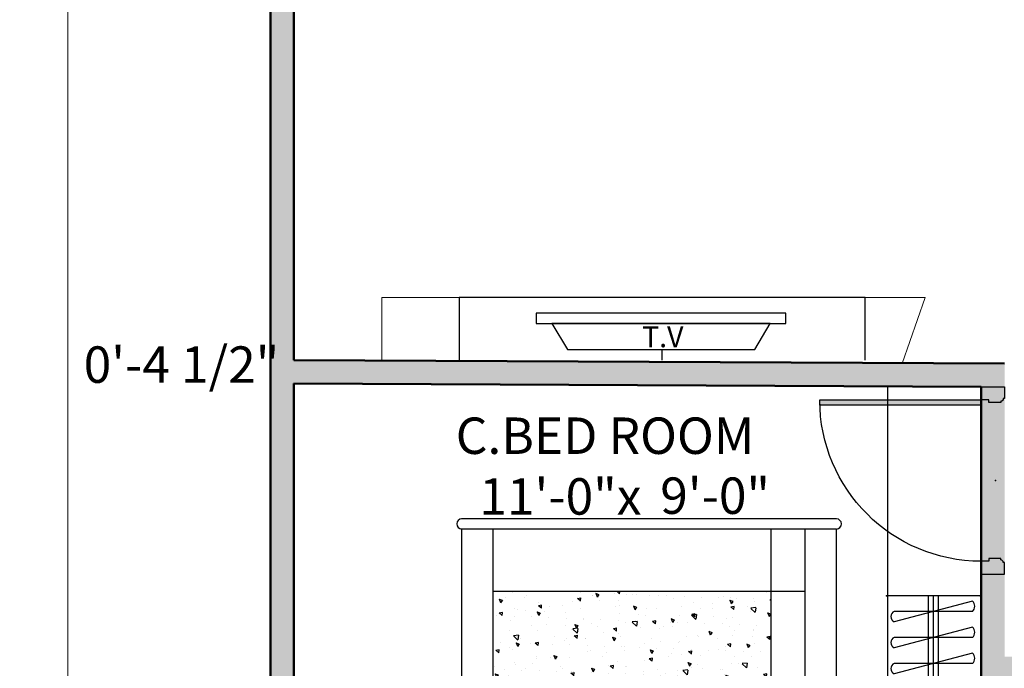
# Model space of a CAD drawing. Units: inches. Extents: x 4508 to 5907, y 877 to 1592.
# Tile 9 of 20: x 5203 to 5392, y 1049 to 1174. Entities that reach past the tile are written whole.
import ezdxf

# ---------------------------------------------------------------- set-up
doc = ezdxf.new("R2010")
doc.units = ezdxf.units.IN
doc.layers.get('DEFPOINTS').update_dxf_attribs({"color": 8})
for name, color, linetype, lineweight in [('A-ANNO-DIMS', 2, 'Continuous', 18), ('A-DOOR', 4, 'Continuous', 25), ('A-FLOR-CASE', 30, 'Continuous', 25), ('A-FURN', 24, 'Continuous', 18), ('A-WALL', 7, 'Continuous', 50), ('A-WALL-PATT', 8, 'Continuous', 13)]:
    doc.layers.add(name, color=color, linetype=linetype, lineweight=lineweight)
doc.layers.add('doors & windows', color=30, linetype='Continuous')
doc.layers.add('furniture', color=24, linetype='Continuous')
doc.styles.get("Standard").update_dxf_attribs({"font": 'arial.ttf'})
doc.dimstyles.new('details', dxfattribs={"dimtxt": 5, "dimasz": 2, "dimexe": 2, "dimexo": 3, "dimgap": 1, "dimtad": 0, "dimdec": 1, "dimzin": 0, "dimdsep": 46, "dimlunit": 4, "dimtxsty": 'Standard', "dimblk": 'ARCHTICK', "dimcen": 3, "dimclrd": 256, "dimclre": 256, "dimclrt": 256, "dimadec": 0, "dimazin": 0, "dimtfac": 0.5, "dimtdec": 1, "dimtofl": 0, "dimtmove": 0, "dimatfit": 3, "dimldrblk": 'CLOSEDBLANK', "dimfxl": 2, "dimtolj": 1, "dimtzin": 0, "dimlwd": -1, "dimlwe": -1, "dimarcsym": 0})
doc.dimstyles.new('text', dxfattribs={"dimtxt": 7, "dimasz": 0, "dimexe": 3, "dimexo": 3, "dimgap": 0, "dimtad": 1, "dimtih": 1, "dimtoh": 1, "dimzin": 3, "dimdsep": 46, "dimlunit": 4, "dimtxsty": 'Standard', "dimblk": 'CLOSEDBLANK', "dimcen": 3, "dimse1": 1, "dimse2": 1, "dimsd1": 1, "dimsd2": 1, "dimclrd": 256, "dimclre": 256, "dimclrt": 256, "dimadec": 0, "dimazin": 0, "dimtfac": 0.5, "dimtofl": 0, "dimtmove": 0, "dimatfit": 3, "dimfxl": 3, "dimtolj": 1, "dimtzin": 0, "dimlwd": -1, "dimlwe": -1, "dimarcsym": 0})

# ---------------------------------------------------------------- blocks, each defined once
blk = doc.blocks.new('_ArchTick')
at = {"color": 0, "linetype": 'ByBlock', "const_width": 0.15}
blk.add_lwpolyline([(-0.5, -0.5), (0.5, 0.5)], dxfattribs=at)
blk = doc.blocks.new('*D77')
at = {"layer": 'A-ANNO-DIMS', "color": 0, "transparency": 16777216}
for p, q in [((5201.49, 1574.7), (5213.97, 1574.7)), ((5211.97, 1574.7), (5211.97, 1255.95)), ((5211.97, 926.7), (5211.97, 1245.46)), ((5201.49, 926.7), (5213.97, 926.7))]:
    blk.add_line(p, q, dxfattribs=at)
at = {"layer": 'DEFPOINTS', "color": 0, "transparency": 16777216}
for p in [(5198.49, 1574.7), (5211.97, 1574.7), (5198.49, 926.7)]:
    blk.add_point(p, dxfattribs=at)
at = {"layer": 'A-ANNO-DIMS', "color": 0, "transparency": 16777216, "xscale": 2, "yscale": 2, "zscale": 2}
for p, rotation in [((5211.97, 1574.7), 90), ((5211.97, 926.7), 270)]:
    blk.add_blockref('_ArchTick', p, dxfattribs=dict(at, rotation=rotation))
at = {"layer": 'A-ANNO-DIMS', "color": 0, "transparency": 16777216, "insert": (5211.97, 1250.7), "char_height": 5, "attachment_point": 5, "rotation": 90}
blk.add_mtext("\\A1;54'", dxfattribs=at)
blk = doc.blocks.new('_ClosedBlank')
at = {"color": 0, "lineweight": -2}
for p, q in [((-1, 0.167), (0, 0)), ((-1, 0.167), (-1, -0.167)), ((0, 0), (-1, -0.167))]:
    blk.add_line(p, q, dxfattribs=at)
blk = doc.blocks.new('*D94')
at = {"layer": 'DEFPOINTS', "color": 0, "transparency": 16777216}
for p in [(5391.9, 1143.25), (5495.4, 1139.55), (5391.9, 1134.58)]:
    blk.add_point(p, dxfattribs=at)
at = {"layer": 'A-ANNO-DIMS', "color": 0, "transparency": 16777216, "insert": (5428.13, 1144.63), "char_height": 7, "attachment_point": 5}
blk.add_mtext('\\A1;         DINING\\P8\'-7{\\H0.5x;\\S1/2;}"x', dxfattribs=at)
blk = doc.blocks.new('tv')
at = {"layer": 'furniture'}
blk.add_line((0, 0), (2, 0), dxfattribs=at)
for points in [[(0, -39), (12, -39), (12, 39), (0, 39)], [(7, 24.19), (7, -23.81), (9, -23.81), (9, 24.19), (7, 24.19)]]:
    blk.add_lwpolyline(points, dxfattribs=at)
blk.add_lwpolyline([(7, -20.81), (7, 21.19), (2, 18.19), (2, -17.81)], close=True, dxfattribs=at)
blk.add_text('T.V', height=4, rotation=270, dxfattribs=at).set_placement((2.46, 3.81))
blk = doc.blocks.new('*D99')
at = {"layer": 'DEFPOINTS', "color": 0, "transparency": 16777216}
for p in [(5336.4, 1294.2), (5345.32, 1294.2), (5334.11, 1108.2)]:
    blk.add_point(p, dxfattribs=at)
at = {"layer": 'A-ANNO-DIMS', "color": 0, "transparency": 16777216, "insert": (5345.32, 1198.7), "char_height": 7, "attachment_point": 5}
blk.add_mtext('\\A1;15\'-6"', dxfattribs=at)
blk = doc.blocks.new('D1')
at = {"layer": 'doors & windows'}
h = blk.add_hatch(dxfattribs=at)
h.set_pattern_fill('DOTS', color=256, scale=2, angle=180, style=0)
h.set_pattern_definition([(180, (-2e-12, -4), (-0.0625, -0.125), [0, -0.125])])
h.paths.add_polyline_path([(2.5, 0), (3.5, 0), (3.5, 30.98, 0.008066), (2.5, 31)])
h = blk.add_hatch(dxfattribs=at)
h.set_pattern_fill('DOTS', color=256, scale=2, angle=180, style=0)
h.set_pattern_definition([(180, (0, -0.5), (-0.0625, -0.125), [0, -0.125])])
h.paths.add_polyline_path([(0, -4.5), (2.25, -4.5), (2.25, -4.25, 0.403966), (2.75, -3.75), (3, -3.75), (3, -1.5), (2.5, -1.5), (2.5, 0), (0, 0)])
h.paths.add_polyline_path([(36, -4.5), (36, 0), (33.5, 0), (33.5, -1.5), (33, -1.5), (33, -3.75), (33.25, -3.75, 0.403966), (33.75, -4.25), (33.75, -4.5)])
for p, q in [((0, 0), (0, -4.5)), ((36, 0), (36, -4.5))]:
    blk.add_line(p, q)
blk.add_lwpolyline([(3.5, 0), (3.5, 31), (2.5, 31), (2.5, 0)], close=True, dxfattribs=at)
for points in [[(3, -3.75), (3, -1.5), (2.5, -1.5), (2.5, 0), (0, 0)], [(33, -3.75), (33, -1.5), (33.5, -1.5), (33.5, 0), (36, 0)], [(0, -4.5), (2.25, -4.5)], [(36, -4.5), (33.75, -4.5)]]:
    blk.add_lwpolyline(points, dxfattribs=at)
for points in [[(2.25, -4.5), (2.25, -4.25, 0.403966), (2.75, -3.75), (3, -3.75)], [(33.75, -4.5), (33.75, -4.25, -0.403966), (33.25, -3.75), (33, -3.75)]]:
    blk.add_lwpolyline(points, format="xyb", dxfattribs=at)
at = {"layer": 'doors & windows', "ltscale": 6}
blk.add_arc((2.5, 0), 31, 0, 90, dxfattribs=at)
at = {"layer": 'doors & windows'}
blk.add_point((18, -2.75), dxfattribs=at)
blk = doc.blocks.new('hangers')
at = {"layer": 'furniture'}
for p, q in [((1, 7.5), (5, -7.5)), ((3, 7.5), (3, -7.5)), ((6, 7.5), (10, -7.5)), ((8, 7.5), (8, -7.5)), ((11, 7.5), (15, -7.5)), ((13, 7.5), (13, -7.5)), ((51, 7.5), (55, -7.5)), ((53, 7.5), (53, -7.5)), ((56, 7.5), (60, -7.5)), ((58, 7.5), (58, -7.5)), ((61, 7.5), (65, -7.5)), ((63, 7.5), (63, -7.5)), ((66, 1), (0, 1)), ((0, 0), (66, 0)), ((0, -1), (66, -1))]:
    blk.add_line(p, q, dxfattribs=at)
for centre, radius, start, end in [((2, 6.62), 1.33, 41.2884, 138.7116), ((7, 6.62), 1.33, 41.2884, 138.7116), ((12, 6.62), 1.33, 41.2884, 138.7116), ((52, 6.62), 1.33, 41.2884, 138.7116), ((57, 6.62), 1.33, 41.2884, 138.7116), ((62, 6.62), 1.33, 41.2884, 138.7116), ((4, -7.08), 1.08, 202.5549, 337.4451), ((9, -7.08), 1.08, 202.5549, 337.4451), ((14, -7.08), 1.08, 202.5549, 337.4451), ((54, -7.08), 1.08, 202.5549, 337.4451), ((59, -7.08), 1.08, 202.5549, 337.4451), ((64, -7.08), 1.08, 202.5549, 337.4451)]:
    blk.add_arc(centre, radius, start, end, dxfattribs=at)
for p in [(0, 9), (66, 9), (0, -9), (66, -9)]:
    blk.add_point(p, dxfattribs=at)
blk.add_text('S H E L V E S', height=4, dxfattribs=at).set_placement((16, -5.52))
blk = doc.blocks.new('bed')
at = {"layer": 'furniture'}
h = blk.add_hatch(dxfattribs=at)
h.set_pattern_fill('AR-CONC', color=256, angle=-90, style=0)
h.set_pattern_definition([(320, (0, 2.38), (-0.6275, -7.1726), [0.75, -8.25]), (265, (0, 2.38), (7.5219, 1.3875), [0.6, -6.6]), (10.451, (-0.052, 1.782), (6.8944, -5.7851), [0.6374, -7.0114]), (316.184, (2, 2.38), (-1.6552, -10.6724), [1.125, -12.375]), (6.636, (1.862, 1.491), (9.7412, -9.3466), [0.9561, -10.5171]), (261.184, (2, 2.38), (9.7412, -9.3466), [0.9, -9.9]), (291, (1.5, 1.38), (-4.0262, -5.96907), [0.75, -8.25]), (236, (1.5, 1.38), (7.2515, -2.43315), [0.6, -6.6]), (341.451, (1.1645, 0.8826), (3.2253, -8.4022), [0.6374, -7.0114]), (307.5, (0, 2.38), (3.32894, -0.1216), [0, -6.52, 0, -6.7, 0, -6.625]), (277.5, (0, 2.38), (3.94412, -2.6307), [0, -3.82, 0, -6.37, 0, -2.525]), (237.5, (0, 4.61), (-0.22555, -5.33822), [0, -2.5, 0, -7.8, 0, -10.35]), (227.5, (0, 5.61), (1.00105, -5.83186), [0, -3.25, 0, -5.18, 0, -7.35])])
h.paths.add_polyline_path([(30.01, -68), (30.01, -26.5, 0.263043), (23.9, -35.15, 0.293424), (-9.18, -26.47, -0.156683), (-23.39, -28.72), (-23.39, -68)])
for p, q in [((0, -3), (0, 0)), ((36.01, -3), (-36.01, -3)), ((-36.01, -5), (-36.01, -80)), ((36.01, -5), (-36.01, -5)), ((0, -8), (0, -5)), ((36.01, -80), (36.01, -5)), ((-31.24, -7.07), (-32.24, -7.07)), ((-3.81, -7.07), (-2.81, -7.07)), ((3.89, -7.07), (2.89, -7.07)), ((31.63, -7.07), (32.63, -7.07)), ((-31.24, -9.07), (-32.24, -9.07)), ((-3.81, -9.07), (-2.81, -9.07)), ((3.89, -9.07), (2.89, -9.07)), ((31.63, -9.07), (32.63, -9.07)), ((-31.24, -11.07), (-32.24, -11.07)), ((-3.81, -11.07), (-2.81, -11.07)), ((3.89, -11.07), (2.89, -11.07)), ((31.63, -11.07), (32.63, -11.07)), ((-31.24, -13.07), (-32.24, -13.07)), ((-3.81, -13.07), (-2.81, -13.07)), ((3.89, -13.07), (2.89, -13.07)), ((31.63, -13.07), (32.63, -13.07)), ((-31.24, -15.07), (-32.24, -15.07)), ((-3.81, -15.07), (-2.81, -15.07)), ((3.89, -15.07), (2.89, -15.07)), ((31.63, -15.07), (32.63, -15.07)), ((-31.24, -17.07), (-32.24, -17.07)), ((-3.81, -17.07), (-2.81, -17.07)), ((3.89, -17.07), (2.89, -17.07)), ((31.63, -17.07), (32.63, -17.07)), ((-31.24, -19.07), (-32.24, -19.07)), ((-3.81, -19.07), (-2.81, -19.07)), ((3.89, -19.07), (2.89, -19.07)), ((31.63, -19.07), (32.63, -19.07)), ((-36.01, -80), (36.01, -80)), ((-36.01, -82), (36.01, -82))]:
    blk.add_line(p, q, dxfattribs=at)
at = {"layer": 'furniture', "ltscale": 5}
blk.add_line((-30.01, -26.66), (-30.01, -80), dxfattribs=at)
at = {"layer": 'furniture', "ltscale": 7}
blk.add_line((30.01, -80), (30.01, -26.5), dxfattribs=at)
at = {"layer": 'furniture', "ltscale": 0.3}
for p, q in [((-23.39, -80), (-23.39, -28.72)), ((-30.01, -68), (30.01, -68))]:
    blk.add_line(p, q, dxfattribs=at)
at = {"layer": 'furniture'}
for centre, radius, start, end in [((-35.95, -4), 1, 93.3831, 266.6169), ((35.95, -4), 1, 273.3831, 86.6169), ((-31.1, -6.57), 0.382, 35.8976, 208.6272), ((-44.44, -13.85), 14.82, 27.1629, 28.6272), ((-46.76, -9.65), 15.72, 357.4804, 9.3956), ((-34.45, -3.51), 9.85, 289.8695, 338.9843), ((-34.45, -3.51), 12.47, 286.0319, 344.1205), ((-26.35, 6.68), 13.76, 251.1782, 273.3982), ((-18.02, -163.6), 156.72, 87.0032, 92.7497), ((-8.03, 2.03), 9.29, 258.896, 294.7184), ((0.25, -8.8), 4.49, 159.0146, 186.273), ((-4.03, -6.67), 0.282, 335.7259, 114.303), ((3.22, -9.94), 7.68, 155.7259, 159.0146), ((4.11, -6.67), 0.282, 65.697, 204.2741), ((-3.14, -9.94), 7.68, 20.9854, 24.2741), ((-0.17, -8.8), 4.49, 353.727, 20.9854), ((8.12, 2.03), 9.29, 245.2816, 281.104), ((18.1, -163.6), 156.72, 87.2503, 92.9968), ((34.54, -3.51), 12.47, 195.8795, 253.9681), ((34.54, -3.51), 9.85, 201.0157, 250.1305), ((26.43, 6.68), 13.76, 266.6018, 288.8218), ((31.18, -6.57), 0.382, 331.3728, 144.1024), ((46.84, -9.65), 15.72, 170.6044, 182.5196), ((44.53, -13.85), 14.82, 151.3728, 152.8371), ((-32.82, -12.44), 28.78, 354.3784, 6.273), ((32.9, -12.44), 28.78, 173.727, 185.6216), ((-28.62, 31.03), 42.31, 266.4836, 266.6487), ((54.88, -13.16), 85.99, 178.1209, 183.3613), ((-54.8, -13.16), 85.99, 356.6387, 1.8791), ((28.7, 31.03), 42.31, 273.3513, 273.5164), ((12.28, -16.11), 16.48, 177.0317, 192.8678), ((-12.19, -16.11), 16.48, 347.1322, 2.9683), ((-34.13, -18.41), 3.18, 342.7809, 3.755), ((34.21, -18.41), 3.18, 176.245, 197.2191), ((-31.05, -19.91), 0.291, 147.6219, 311.9343), ((-33.2, -18.55), 2.25, 327.6219, 339.2246), ((-24.4, -58.01), 38.42, 93.5164, 99.6766), ((-24.52, -56.06), 36.48, 86.4836, 93.5164), ((-18.49, 70.49), 90.23, 267.5921, 273.6329), ((-10.31, -44.95), 25.52, 75.952, 95.5452), ((-3.95, -19.99), 0.265, 231.9005, 52.8902), ((4.03, -19.99), 0.265, 127.1098, 308.0995), ((7.57, -34.68), 14.87, 87.3976, 103.1191), ((11.44, -34.81), 15.32, 84.694, 102.0355), ((18.57, 70.49), 90.23, 266.3671, 272.4079), ((24.6, -56.06), 36.48, 86.4836, 93.5164), ((24.48, -58.01), 38.42, 80.3234, 86.4836), ((31.13, -19.91), 0.291, 228.0657, 32.3781), ((33.28, -18.55), 2.25, 200.7754, 212.3781), ((-19.79, -5.47), 23.53, 226.4061, 297.4441), ((12.51, -69.71), 48.38, 60.9345, 116.3227), ((0.6, -56.57), 31.65, 42.5874, 108.5034), ((34.61, -36.23), 10.76, 101.1719, 174.259), ((-35.95, -81), 1, 93.3831, 266.6169), ((35.95, -81), 1, 273.3831, 86.6169)]:
    blk.add_arc(centre, radius, start, end, dxfattribs=at)
blk = doc.blocks.new('*D100')
at = {"layer": 'DEFPOINTS', "color": 0, "transparency": 16777216}
for p in [(5344.94, 1103.25), (5336.34, 995.27), (5340.97, 995.27)]:
    blk.add_point(p, dxfattribs=at)
at = {"layer": 'A-ANNO-DIMS', "color": 0, "transparency": 16777216, "insert": (5336.34, 1082.13), "char_height": 7, "attachment_point": 5}
blk.add_mtext('\\A1;9\'-0"', dxfattribs=at)
blk = doc.blocks.new('*D101')
at = {"layer": 'DEFPOINTS', "color": 0, "transparency": 16777216}
for p in [(5387.45, 1078.35), (5255.4, 1067.28), (5387.45, 1052.04)]:
    blk.add_point(p, dxfattribs=at)
at = {"layer": 'A-ANNO-DIMS', "color": 0, "transparency": 16777216, "insert": (5306.62, 1087.82), "char_height": 7, "attachment_point": 5}
blk.add_mtext('\\A1;        C.BED ROOM\\P11\'-0"x', dxfattribs=at)
blk = doc.blocks.new('*D190')
at = {"layer": 'DEFPOINTS', "color": 0, "transparency": 16777216}
for p in [(5216.35, 1108.2), (5255.4, 1108.2), (5255.4, 1103.7)]:
    blk.add_point(p, dxfattribs=at)
at = {"layer": 'A-ANNO-DIMS', "transparency": 16777216, "insert": (5233.81, 1107.32), "char_height": 7, "attachment_point": 5}
blk.add_mtext('\\A1;0\'-4 1/2"', dxfattribs=at)

msp = doc.modelspace()

# ---------------------------------------------------------------- hatches: boundary and pattern name
at = {"layer": 'A-WALL-PATT'}
h = msp.add_hatch(color=256, dxfattribs=at)
h.dxf.hatch_style = 1
h.paths.add_polyline_path([(5529.903, 1303.204), (5388.02, 1303.204), (5388.02, 1294.204), (5391.903, 1294.204), (5391.903, 1205.704), (5396.403, 1205.704), (5396.403, 1294.204), (5489.403, 1294.204), (5489.403, 1256.139), (5493.903, 1256.139), (5493.903, 1294.204), (5529.903, 1294.204)], flags=17)
h.paths.add_polyline_path([(5346.02, 1303.204), (5322.903, 1303.204), (5322.903, 1321.388), (5313.903, 1321.388), (5313.903, 1303.204), (5259.903, 1303.204), (5259.903, 1381.204), (5313.903, 1381.204), (5313.903, 1359.674), (5322.903, 1359.674), (5322.903, 1381.204), (5338.979, 1381.204), (5338.979, 1390.204), (5331.903, 1390.204), (5331.903, 1442.704), (5255.403, 1442.704), (5255.403, 1570.204), (5387.403, 1570.204), (5387.403, 1541.271), (5391.903, 1541.271), (5391.903, 1570.204), (5483.403, 1570.204), (5483.403, 1498.204), (5391.903, 1498.204), (5391.903, 1509.559), (5387.403, 1509.559), (5387.403, 1390.204), (5380.979, 1390.204), (5380.979, 1381.204), (5387.403, 1381.204), (5529.903, 1381.204), (5529.903, 1498.204), (5487.903, 1498.204), (5487.903, 1570.204), (5529.903, 1570.204), (5529.903, 1574.704), (5250.903, 1574.704), (5250.903, 991.204), (5310.903, 991.204), (5310.903, 926.704), (5529.903, 926.704), (5529.903, 1210.204), (5525.403, 1210.204), (5525.403, 1103.704), (5499.903, 1103.704), (5499.903, 1210.204), (5493.903, 1210.204), (5493.903, 1256.139), (5489.403, 1256.139), (5489.403, 1210.204), (5461.584, 1210.204), (5461.584, 1205.704), (5495.403, 1205.704), (5495.403, 1103.704), (5436.903, 1103.704), (5436.903, 1051.204), (5391.954, 1051.204), (5391.954, 1103.03), (5391.954, 1107.53), (5255.403, 1108.204), (5255.403, 1294.204), (5346.02, 1294.204)])
h.paths.add_polyline_path([(5255.403, 1390.204), (5255.403, 1398.204), (5255.403, 1438.204), (5257.903, 1438.204), (5258.903, 1438.204), (5327.403, 1438.204), (5327.403, 1390.204), (5325.903, 1390.204)], flags=16)
h.paths.add_polyline_path([(5288.757, 1390.704), (5288.757, 1390.204), (5292.173, 1390.204), (5292.173, 1390.704)], flags=0)
h.paths.add_polyline_path([(5289.965, 1391.606), (5289.965, 1396.645), (5289.903, 1396.645), (5289.903, 1397.319), (5288.849, 1398.862), (5288.849, 1398.8), (5288.983, 1398.748), (5288.983, 1399.204), (5289.091, 1399.204), (5292.081, 1399.204), (5292.081, 1398.665), (5291.946, 1398.665), (5291.027, 1397.319), (5291.027, 1396.645), (5290.965, 1396.645), (5290.965, 1391.606)], flags=0)
h.paths.add_polyline_path([(5288.849, 1399.069, 2.6374395), (5289.056, 1398.835), (5289.117, 1399.087, 0.9346155)], flags=0)
h.paths.add_polyline_path([(5290.061, 1398.665), (5290.061, 1399.204), (5290.038, 1398.975)], flags=0)
h.paths.add_polyline_path([(5291.946, 1398.934, -1), (5291.946, 1398.665)], flags=0)
h.paths.add_polyline_path([(5289.414, 1398.967), (5289.414, 1399.204), (5289.63, 1399.204), (5289.63, 1398.363), (5290.051, 1397.184), (5290.76, 1397.184), (5290.869, 1398.665), (5290.869, 1399.204), (5290.815, 1398.665), (5290.815, 1399.204), (5291.462, 1399.204), (5291.462, 1398.816), (5290.879, 1397.184), (5290.051, 1397.184)], flags=0)
h.paths.add_polyline_path([(5273.903, 1392.056), (5269.591, 1392.056, 0.0901028), (5265.544, 1392.842), (5265.511, 1392.034, -0.3516542), (5265.903, 1391.546, -1), (5264.903, 1391.546, -0.3042165), (5265.213, 1392.008), (5265.167, 1392.84, 0.0880132), (5261.215, 1392.056), (5256.903, 1392.056), (5256.903, 1398.704, -0.4142136), (5259.403, 1401.204), (5271.403, 1401.204, -0.4142136), (5273.903, 1398.704)], flags=0)
h.paths.add_polyline_path([(5263.726, 1395.073, -1), (5267.08, 1395.073, -1)], flags=0)
h.paths.add_polyline_path([(5264.434, 1395.073, -0.695521), (5265.153, 1395.073, -1.1408699), (5265.403, 1395.585, -0.7522125), (5265.403, 1396.25, 0.3674806)], flags=0)
h.paths.add_polyline_path([(5265.153, 1394.399, -1), (5265.653, 1394.399, -1)], flags=0)
h.paths.add_polyline_path([(5265.905, 1395.077, -1), (5266.405, 1395.077, -1)], flags=0)
h.paths.add_polyline_path([(5307.994, 1403.113, -1), (5307.994, 1417.295), (5318.794, 1417.295, -0.4142136), (5319.794, 1416.295), (5320.794, 1416.295, -0.4142136), (5321.794, 1417.295), (5324.903, 1417.295, -0.4142136), (5325.903, 1416.295), (5325.903, 1404.113, -0.4142136), (5324.903, 1403.113), (5321.794, 1403.113, -0.4142136), (5320.794, 1404.113), (5319.794, 1404.113, -0.4142136), (5318.794, 1403.113)], flags=0)
h.paths.add_polyline_path([(5307.836, 1405.113, -1), (5307.836, 1415.295), (5315.591, 1415.295, -0.4142136), (5317.532, 1413.353), (5317.532, 1407.054, -0.4142136), (5315.591, 1405.113)], flags=0)
h.paths.add_polyline_path([(5312.032, 1408.204, -1), (5312.032, 1412.204), (5315.032, 1412.204, -0.4142136), (5316.032, 1411.204), (5316.032, 1409.204, -0.4142136), (5315.032, 1408.204)], flags=0)
h.paths.add_polyline_path([(5391.903, 1385.704), (5391.903, 1493.704), (5525.403, 1493.704), (5525.403, 1385.704)], flags=16)
h.paths.add_polyline_path([(5422.641, 1390.704), (5422.641, 1465.704, -0.9426302), (5422.641, 1467.704), (5494.547, 1467.704, -1), (5494.665, 1465.704), (5494.665, 1390.704, -0.9426302), (5494.665, 1388.704), (5422.759, 1388.704, -1)], flags=0)
h.paths.add_polyline_path([(5427.52, 1395.749, -0.0238564), (5427.614, 1403.949, 0.0884332), (5427.476, 1405.056, 0.0506693), (5427.273, 1405.463, -0.8716827), (5427.713, 1405.835, 0.0268855), (5431.815, 1405.361, 0.0306964), (5436.289, 1405.361, -0.0263641), (5445.798, 1405.259, 0.075811), (5450.408, 1405.53, 0.0687062), (5454.457, 1405.903, -1.0086747), (5454.781, 1405.482, 0.0692081), (5454.389, 1400.959, -0.0519468), (5454.356, 1394.996, 0.1195012), (5454.627, 1392.895, 0.0143508), (5454.796, 1392.489, -0.6962059), (5454.42, 1392.118, 0.1574808), (5448.747, 1392.794, -0.025536), (5432.749, 1392.774, 0.0920085), (5427.781, 1392.048, -0.9384848), (5427.137, 1392.455, 0.0063894), (5427.314, 1392.79, 0.0472995)], flags=0)
h.paths.add_polyline_path([(5426.125, 1411.372, 0.0617649), (5428.641, 1412.201), (5428.641, 1465.704), (5488.665, 1465.704), (5488.665, 1412.363, 0.2363822), (5467.6, 1412.052, -0.2252042)], flags=0)
h.paths.add_polyline_path([(5391.903, 1490.204), (5391.903, 1491.204), (5422.903, 1491.204), (5422.903, 1490.204)], flags=0)
h.paths.add_polyline_path([(5462.545, 1392.771, 0.1270318), (5462.866, 1394.996, -0.0519468), (5462.832, 1400.959, 0.0692081), (5462.441, 1405.482, -1.0086747), (5462.765, 1405.903, 0.0857004), (5471.424, 1405.259, -0.0263641), (5480.932, 1405.361, 0.0306964), (5485.407, 1405.361, 0.0268855), (5489.509, 1405.835, -0.8716827), (5489.949, 1405.463, 0.0506693), (5489.746, 1405.056, 0.0884332), (5489.608, 1403.949, -0.0238564), (5489.702, 1395.749, 0.0472995), (5489.908, 1392.79, 0.0063894), (5490.085, 1392.455, -0.9384848), (5489.441, 1392.048, 0.0920085), (5484.473, 1392.774, -0.025536), (5468.475, 1392.794, 0.1574808), (5462.802, 1392.118, -0.6962059), (5462.426, 1392.489, 0.0100173), (5462.546, 1392.771)], flags=0)
h.paths.add_polyline_path([(5387.454, 1103.03), (5387.454, 1100.53), (5387.454, 1099.53), (5387.454, 995.03), (5387.454, 991.204), (5391.954, 991.204), (5391.954, 1046.704), (5525.403, 1046.704), (5525.403, 931.182), (5391.954, 930.53), (5391.954, 960.53), (5387.454, 960.53), (5387.454, 930.53), (5315.403, 930.53), (5315.403, 991.204), (5323.403, 991.204), (5387.454, 991.204), (5387.454, 995.03), (5255.403, 995.704), (5255.403, 1103.704)], flags=16)
h.paths.add_polyline_path([(5379.264, 1062.889), (5379.264, 1060.156), (5385.764, 1061.889, -0.4526903), (5385.764, 1059.889), (5379.264, 1059.889), (5379.264, 1055.156), (5385.764, 1056.889, -0.4526903), (5385.764, 1054.889), (5379.264, 1054.889), (5379.264, 1050.156), (5385.764, 1051.889, -0.4526903), (5385.764, 1049.889), (5379.264, 1049.889), (5379.264, 1010.156), (5385.764, 1011.889, -0.4526903), (5385.764, 1009.889), (5379.264, 1009.889), (5379.264, 1005.156), (5385.764, 1006.889, -0.4526903), (5385.764, 1004.889), (5379.264, 1004.889), (5379.264, 1000.156), (5385.764, 1001.889, -0.4526903), (5385.764, 999.889), (5378.264, 999.889), (5370.764, 997.889, -0.6674863), (5370.764, 999.889), (5377.264, 999.889), (5377.264, 1004.623), (5370.764, 1002.889, -0.6674863), (5370.764, 1004.889), (5377.264, 1004.889), (5377.264, 1009.623), (5370.764, 1007.889, -0.6674863), (5370.764, 1009.889), (5377.264, 1009.889), (5377.264, 1049.623), (5370.764, 1047.889, -0.6674863), (5370.764, 1049.889), (5377.264, 1049.889), (5377.264, 1054.623), (5370.764, 1052.889, -0.6674863), (5370.764, 1054.889), (5377.264, 1054.889), (5377.264, 1059.623), (5370.764, 1057.889, -0.6674863), (5370.764, 1059.889), (5377.264, 1059.889), (5377.264, 1062.889)], flags=0)
h.paths.add_polyline_path([(5287.641, 1000.704), (5359.665, 1000.704), (5359.665, 1018.212, 0.3202856), (5332.6, 1022.052, -0.246494), (5287.641, 1023.128)], flags=0)
h.paths.add_polyline_path([(5359.547, 1077.704, -1), (5359.665, 1075.704), (5353.665, 1075.704), (5353.665, 1063.704), (5293.641, 1063.704), (5293.641, 1075.704), (5287.759, 1075.704, -1), (5287.641, 1077.704)], flags=0)
h.paths.add_polyline_path([(5441.403, 1099.204), (5525.403, 1099.204), (5525.403, 1051.204), (5441.403, 1051.204), (5441.403, 1059.204)], flags=16)
h.paths.add_polyline_path([(5441.403, 1096.704), (5466.403, 1096.704), (5466.403, 1095.704), (5441.403, 1095.704)], flags=0)
h.paths.add_polyline_path([(5445.403, 1062.204), (5457.403, 1062.204, -0.4142136), (5459.903, 1059.704), (5459.903, 1053.056), (5455.591, 1053.056, 0.0901028), (5451.544, 1053.842), (5451.511, 1053.034, -0.3516542), (5451.903, 1052.546, -1), (5450.903, 1052.546, -0.3042165), (5451.213, 1053.008), (5451.167, 1053.84, 0.0880132), (5447.215, 1053.056), (5442.903, 1053.056), (5442.903, 1059.704, -0.4142136)], flags=0)
h.paths.add_polyline_path([(5453.08, 1056.073, -1), (5449.726, 1056.073, -1)], flags=0)
h.paths.add_polyline_path([(5292.713, 1015.835, 0.0268855), (5296.815, 1015.361, 0.0306964), (5301.289, 1015.361, -0.0263641), (5310.798, 1015.259, 0.075811), (5315.408, 1015.53, 0.0687062), (5319.457, 1015.903, -1.0086747), (5319.781, 1015.482, 0.0692081), (5319.389, 1010.959, -0.0519468), (5319.356, 1004.996, 0.1195012), (5319.627, 1002.895, 0.0143508), (5319.796, 1002.489, -0.6962059), (5319.42, 1002.118, 0.1574808), (5313.747, 1002.794, -0.025536), (5297.749, 1002.774, 0.0920085), (5292.781, 1002.048, -0.9384848), (5292.137, 1002.455, 0.0063894), (5292.314, 1002.79, 0.0472995), (5292.52, 1005.749, -0.0238564), (5292.614, 1013.949, 0.0884332), (5292.476, 1015.056, 0.0506693), (5292.273, 1015.463, -0.8716827)], flags=0)
h.paths.add_polyline_path([(5450.434, 1056.073, -0.695521), (5451.153, 1056.073, -1.1408699), (5451.403, 1056.585, -0.7522125), (5451.403, 1057.25, 0.3674806)], flags=0)
h.paths.add_polyline_path([(5327.765, 1015.903, 0.0857004), (5336.424, 1015.259, -0.0263641), (5345.932, 1015.361, 0.0306964), (5350.407, 1015.361, 0.0268855), (5354.509, 1015.835, -0.8716827), (5354.949, 1015.463, 0.0506693), (5354.746, 1015.056, 0.0884332), (5354.608, 1013.949, -0.0238564), (5354.702, 1005.749, 0.0472995), (5354.908, 1002.79, 0.0063894), (5355.085, 1002.455, -0.9384848), (5354.441, 1002.048, 0.0920085), (5349.473, 1002.774, -0.025536), (5333.475, 1002.794, 0.1574808), (5327.802, 1002.118, -0.6962059), (5327.426, 1002.489, 0.0100173), (5327.546, 1002.771), (5327.545, 1002.771, 0.1270318), (5327.866, 1004.996, -0.0519468), (5327.832, 1010.959, 0.0692081), (5327.441, 1015.482, -1.0086747)], flags=0)
h.paths.add_polyline_path([(5452.405, 1056.077, -1), (5451.905, 1056.077, -1)], flags=0)
h.paths.add_polyline_path([(5451.653, 1055.399, -1), (5451.153, 1055.399, -1)], flags=0)
h.paths.add_polyline_path([(5472.958, 1051.704), (5472.958, 1051.204), (5476.374, 1051.204), (5476.374, 1051.704)], flags=0)
h.paths.add_polyline_path([(5476.282, 1060.204), (5476.282, 1059.665), (5476.147, 1059.665), (5475.228, 1058.319), (5475.228, 1057.645), (5475.166, 1052.606), (5474.166, 1052.606), (5474.166, 1057.645), (5474.104, 1057.645), (5474.104, 1058.319), (5473.05, 1059.862), (5473.05, 1059.8), (5473.184, 1059.748), (5473.184, 1060.204), (5473.292, 1060.204)], flags=0)
h.paths.add_polyline_path([(5473.05, 1060.069, 2.6374395), (5473.257, 1059.835), (5473.318, 1060.087, 0.9346155)], flags=0)
h.paths.add_polyline_path([(5473.831, 1060.204), (5473.831, 1059.363), (5474.252, 1058.184), (5474.371, 1058.184), (5474.262, 1059.665), (5474.262, 1060.204)], flags=0)
h.paths.add_polyline_path([(5475.501, 1060.204), (5475.501, 1059.363), (5475.555, 1059.514), (5475.555, 1060.204)], flags=0)
h.paths.add_polyline_path([(5474.855, 1060.204), (5474.908, 1060.127), (5474.908, 1060.204), (5474.855, 1059.665)], flags=0)
h.paths.add_polyline_path([(5476.147, 1059.934, -1), (5476.147, 1059.665)], flags=0)
h.paths.add_polyline_path([(5474.693, 1060.204), (5475.178, 1059.511), (5475.178, 1060.204), (5475.285, 1059.934), (5475.285, 1060.204), (5475.178, 1059.665), (5475.178, 1060.204), (5475.07, 1059.665), (5475.07, 1060.204), (5474.962, 1059.665), (5474.962, 1060.204), (5474.693, 1059.306)], flags=0)
h.paths.add_polyline_path([(5474.747, 1060.204), (5474.37, 1059.45), (5474.37, 1060.204), (5474.424, 1060.096), (5474.424, 1060.204), (5474.747, 1059.665)], flags=0)
h.paths.add_polyline_path([(5476.04, 1059.665), (5476.04, 1060.204), (5476.094, 1059.665), (5476.094, 1060.204)], flags=0)
h.paths.add_polyline_path([(5505.994, 1082.295), (5516.794, 1082.295, -0.4142136), (5517.794, 1081.295), (5518.794, 1081.295, -0.4142136), (5519.794, 1082.295), (5522.903, 1082.295, -0.4142136), (5523.903, 1081.295), (5523.903, 1069.113, -0.4142136), (5522.903, 1068.113), (5519.794, 1068.113, -0.4142136), (5518.794, 1069.113), (5517.794, 1069.113, -0.4142136), (5516.794, 1068.113), (5505.994, 1068.113, -1)], flags=0)
h.paths.add_polyline_path([(5505.836, 1080.295), (5513.591, 1080.295, -0.4142136), (5515.532, 1078.353), (5515.532, 1072.054, -0.4142136), (5513.591, 1070.113), (5505.836, 1070.113, -1)], flags=0)
h.paths.add_polyline_path([(5520.403, 963.695), (5520.403, 1035.72), (5502.895, 1035.72, 0.3202856), (5499.055, 1008.654, -0.246494), (5497.978, 963.695)], flags=0)
h.paths.add_polyline_path([(5445.403, 1035.72), (5445.403, 1029.72), (5457.403, 1029.72), (5457.403, 969.695), (5445.403, 969.695), (5445.403, 963.814, -1), (5443.403, 963.695), (5443.403, 1035.602, -1)], flags=0)
h.paths.add_polyline_path([(5510.032, 1077.204), (5513.032, 1077.204, -0.4142136), (5514.032, 1076.204), (5514.032, 1074.204, -0.4142136), (5513.032, 1073.204), (5510.032, 1073.204, -1)], flags=0)
h.paths.add_polyline_path([(5317.255, 989.704), (5323.903, 989.704, -0.4142136), (5326.403, 987.204), (5326.403, 975.204, -0.4142136), (5323.903, 972.704), (5317.255, 972.704), (5317.255, 977.016, 0.0901028), (5318.041, 981.063), (5317.233, 981.096, -0.8964437), (5316.245, 981.204, -0.8220123), (5317.207, 981.394), (5318.04, 981.44, 0.0880132), (5317.255, 985.392)], flags=0)
h.paths.add_polyline_path([(5321.949, 981.204, -1), (5318.594, 981.204, -1)], flags=0)
h.paths.add_polyline_path([(5362.454, 988.03), (5387.454, 988.03), (5387.454, 990.53), (5391.954, 990.53), (5391.704, 988.289, -0.4090807), (5391.204, 987.78), (5391.204, 987.53), (5388.954, 987.53), (5388.954, 988.03), (5387.454, 988.03), (5387.454, 987.03), (5362.474, 987.03, 0.4025427), (5387.454, 963.03), (5388.954, 963.03), (5388.954, 963.53), (5391.195, 963.28, -0.4142136), (5391.704, 962.771), (5391.954, 960.53), (5391.954, 962.78), (5391.704, 962.78, 0.4090807), (5391.195, 963.28), (5388.954, 963.53), (5388.954, 963.03), (5387.454, 963.03, -0.4025427), (5362.474, 987.03), (5362.454, 987.03)], flags=0)
h.paths.add_polyline_path([(5321.285, 981.204, -0.6555366), (5320.522, 981.204, -1.1195284), (5320.275, 980.701, -1.3500746), (5320.279, 980.026, 0.3749463)], flags=0)
h.paths.add_polyline_path([(5320.022, 981.923, -1), (5320.522, 981.923, -1)], flags=0)
h.paths.add_polyline_path([(5319.348, 981.204, -1), (5319.848, 981.204, -1)], flags=0)
h.paths.add_polyline_path([(5507.157, 1030.662, -0.0238564), (5515.358, 1030.756, 0.0472995), (5518.317, 1030.962, 0.0063894), (5518.652, 1031.139, -0.9384848), (5519.059, 1030.495, 0.0920085), (5518.333, 1025.527, -0.025536), (5518.313, 1009.53, 0.1574808), (5518.989, 1003.857, -0.6962059), (5518.618, 1003.48, 0.0100173), (5518.335, 1003.601), (5518.335, 1003.6, 0.1270318), (5516.111, 1003.921, -0.0519468), (5510.148, 1003.887, 0.0692081), (5505.624, 1003.495, -1.0086747), (5505.204, 1003.819, 0.0857004), (5505.848, 1012.479, -0.0263641), (5505.746, 1021.987, 0.0306964), (5505.746, 1026.462, 0.0268855), (5505.272, 1030.563, -0.8716827), (5505.644, 1031.004, 0.0506693), (5506.051, 1030.801, 0.0884332)], flags=0)
h.paths.add_polyline_path([(5368.045, 945.621), (5378.845, 945.621, -0.4142136), (5379.845, 944.621), (5380.845, 944.621, -0.4142136), (5381.845, 945.621), (5384.954, 945.621, -0.4142136), (5385.954, 944.621), (5385.954, 932.439, -0.4142136), (5384.954, 931.439), (5381.845, 931.439, -0.4142136), (5380.845, 932.439), (5379.845, 932.439, -0.4142136), (5378.845, 931.439), (5368.045, 931.439, -1)], flags=0)
h.paths.add_polyline_path([(5327.31, 931.03), (5327.31, 930.53), (5330.726, 930.53), (5330.726, 931.03)], flags=0)
h.paths.add_polyline_path([(5330.634, 939.53), (5330.634, 938.991), (5330.499, 938.991), (5329.579, 937.645), (5329.579, 936.971), (5329.518, 936.971), (5329.518, 931.933), (5328.518, 931.933), (5328.518, 936.971), (5328.456, 936.971), (5328.456, 937.645), (5327.402, 939.189), (5327.402, 939.126), (5327.536, 939.074), (5327.536, 939.53), (5327.644, 939.53)], flags=0)
h.paths.add_polyline_path([(5327.402, 939.395, 2.6374395), (5327.609, 939.161), (5327.67, 939.414, 0.9346155)], flags=0)
h.paths.add_polyline_path([(5328.021, 939.142), (5328.021, 939.53), (5327.967, 939.53), (5327.967, 939.293)], flags=0)
h.paths.add_polyline_path([(5328.614, 939.53), (5328.614, 938.991), (5328.723, 937.51), (5329.313, 937.51), (5329.422, 938.991), (5329.422, 939.53), (5329.368, 938.991), (5329.368, 939.53)], flags=0)
h.paths.add_polyline_path([(5329.853, 939.53), (5329.853, 938.689), (5329.907, 938.84), (5329.907, 939.53)], flags=0)
h.paths.add_polyline_path([(5330.499, 939.261, -1), (5330.499, 938.991)], flags=0)
h.paths.add_polyline_path([(5367.887, 943.621), (5375.641, 943.621, -0.4142136), (5377.583, 941.68), (5377.583, 935.38, -0.4142136), (5375.641, 933.439), (5367.887, 933.439, -1)], flags=0)
h.paths.add_polyline_path([(5509.267, 947.14), (5509.267, 939.64), (5511.267, 932.14, -0.4526903), (5509.267, 932.14), (5509.267, 938.64), (5504.534, 938.64), (5506.267, 932.14, -0.4526903), (5504.267, 932.14), (5504.267, 938.64), (5499.534, 938.64), (5501.267, 932.14, -0.4526903), (5499.267, 932.14), (5499.267, 938.64), (5459.534, 938.64), (5461.267, 932.14, -0.4526903), (5459.267, 932.14), (5459.267, 938.64), (5454.534, 938.64), (5456.267, 932.14, -0.4526903), (5454.267, 932.14), (5454.267, 938.64), (5449.534, 938.64), (5451.267, 932.14, -0.4526903), (5449.267, 932.14), (5449.267, 939.64), (5447.267, 947.14, -0.3030853), (5448.267, 947.808), (5508.266, 947.808, -0.3032033)], flags=0)
h.paths.add_polyline_path([(5510.148, 995.444, -0.0519468), (5516.111, 995.41, 0.1195012), (5518.212, 995.681, 0.0143508), (5518.618, 995.851, -0.6962059), (5518.989, 995.474, 0.1574808), (5518.313, 989.801, -0.025536), (5518.333, 973.804, 0.0920085), (5519.059, 968.836, -0.9384848), (5518.652, 968.192, 0.0063894), (5518.317, 968.369, 0.0472995), (5515.358, 968.575, -0.0238564), (5507.157, 968.669, 0.0884332), (5506.051, 968.531, 0.0506693), (5505.644, 968.327, -0.8716827), (5505.272, 968.768, 0.0268855), (5505.746, 972.869, 0.0306964), (5505.746, 977.344, -0.0263641), (5505.848, 986.852, 0.075811), (5505.576, 991.462, 0.0687062), (5505.204, 995.512, -1.0086747), (5505.624, 995.836, 0.0692081)], flags=0)
h.paths.add_polyline_path([(5372.083, 940.53), (5375.083, 940.53, -0.4142136), (5376.083, 939.53), (5376.083, 937.53, -0.4142136), (5375.083, 936.53), (5372.083, 936.53, -1)], flags=0)
h.paths.add_polyline_path([(5409.258, 1465.643), (5487.738, 1465.643), (5487.738, 1492.394), (5409.258, 1492.394)], flags=8)
h.paths.add_polyline_path([(5463.574, 1465.103), (5486.546, 1465.103), (5486.546, 1479.528), (5463.574, 1479.528)], flags=8)
h.paths.add_polyline_path([(5248.665, 1406.171), (5299.981, 1406.171), (5299.981, 1432.34), (5248.665, 1432.34)], flags=9)
h.paths.add_polyline_path([(5287.471, 1405.121), (5310.443, 1405.121), (5310.443, 1419.546), (5287.471, 1419.546)], flags=8)
h.paths.add_polyline_path([(5371.637, 1047.927), (5371.637, 1010.764), (5377.841, 1010.764), (5377.841, 1047.927)], flags=8)
h.paths.add_polyline_path([(5324.882, 1074.869), (5347.854, 1074.869), (5347.854, 1089.294), (5324.882, 1089.294)], flags=8)
h.paths.add_polyline_path([(5262.863, 1074.665), (5351.123, 1074.665), (5351.123, 1100.833), (5262.863, 1100.833)], flags=8)
h.paths.add_polyline_path([(5307.238, 938.814), (5363.988, 938.814), (5363.988, 964.982), (5307.238, 964.982)], flags=24)
h.paths.add_polyline_path([(5348.837, 937.997), (5371.809, 937.997), (5371.809, 952.422), (5348.837, 952.422)], flags=8)
h.paths.add_polyline_path([(5432.497, 1066.695), (5489.247, 1066.695), (5489.247, 1092.863), (5432.497, 1092.863)], flags=24)
h.paths.add_polyline_path([(5473.52, 1065.943), (5496.492, 1065.943), (5496.492, 1080.368), (5473.52, 1080.368)], flags=8)
h.paths.add_polyline_path([(5451.783, 984.266), (5480.194, 984.266), (5480.194, 998.691), (5451.783, 998.691)], flags=8)
h.paths.add_polyline_path([(5392.211, 983.632), (5481.554, 983.632), (5481.554, 1010.383), (5392.211, 1010.383)], flags=8)
h.paths.add_polyline_path([(5497.304, 946.267), (5460.142, 946.267), (5460.142, 940.062), (5497.304, 940.062)], flags=8)

# ---------------------------------------------------------------- linework, layer by layer
at = {"layer": 'A-FLOR-CASE'}
for p, q in [((5369.454, 1103.03), (5369.454, 995.03)), ((5387.264, 1062.889), (5369.454, 1062.889))]:
    msp.add_line(p, q, dxfattribs=at)
at = {"layer": 'A-FURN'}
msp.add_lwpolyline([(5372.26, 1107.53), (5376.709, 1120.204), (5272.309, 1120.204), (5272.309, 1108.204)], dxfattribs=at)
at = {"layer": 'A-WALL'}
for p, q in [((5250.903, 926.704), (5250.903, 1574.704)), ((5255.403, 1108.204), (5255.403, 1294.204)), ((5255.403, 1108.204), (5391.954, 1107.53)), ((5255.403, 1103.704), (5387.454, 1103.03)), ((5255.403, 995.704), (5255.403, 1103.704)), ((5387.454, 1103.03), (5387.454, 995.03))]:
    msp.add_line(p, q, dxfattribs=at)

# ---------------------------------------------------------------- block references
at = {"layer": 'A-DOOR', "xscale": -1, "rotation": 90}
msp.add_blockref('D1', (5387.454, 1103.03), dxfattribs=at)
at = {"layer": 'A-FURN'}
for name, p, rotation in [('tv', (5326.138, 1108.204), 90), ('bed', (5323.653, 995.704), 180), ('hangers', (5378.264, 1062.889), 270)]:
    msp.add_blockref(name, p, dxfattribs=dict(at, rotation=rotation))

# ---------------------------------------------------------------- dimensions: what is measured, and where the dimension line sits
at = {"layer": 'A-ANNO-DIMS'}
for base, p1, p2, dimstyle, override, picture, middle in [((5211.971, 1574.704), (5198.492, 926.704), (5198.492, 1574.704), 'details', {"dimclrd": 0, "dimclre": 0, "dimclrt": 0}, '*D77', (5211.971, 1250.704)), ((5216.353, 1108.204), (5255.403, 1103.704), (5255.403, 1108.204), 'text', {"dimdec": 1, "dimlfac": 1, "dimrnd": 0, "dimzin": 1, "dimdsep": 46, "dimlunit": 4, "dimfrac": 2}, '*D190', (5233.812, 1107.323))]:
    dim = msp.add_linear_dim(base=base, p1=p1, p2=p2, angle=90, dimstyle=dimstyle, override=override, dxfattribs=at)
    dim.commit()
    dim.dimension.update_dxf_attribs({"geometry": picture, "text_midpoint": middle})
for base, p1, p2, picture, middle in [((5345.321, 1294.204), (5334.11, 1108.204), (5336.404, 1294.204), '*D99', (5345.321, 1198.701)), ((5336.342, 995.267), (5344.937, 1103.247), (5340.973, 995.267), '*D100', (5336.342, 1082.132))]:
    dim = msp.add_linear_dim(base=base, p1=p1, p2=p2, angle=90, dimstyle='text', override={"dimclrd": 0, "dimclre": 0, "dimclrt": 0}, dxfattribs=at)
    dim.commit()
    dim.dimension.update_dxf_attribs({"geometry": picture, "text_midpoint": middle, "dimtype": 160})
dim = msp.add_linear_dim(base=(5391.903, 1134.578), p1=(5495.403, 1139.552), p2=(5391.903, 1143.255), angle=180, text='         DINING\\P<>x', dimstyle='text', override={"dimclrd": 0, "dimclre": 0, "dimclrt": 0}, dxfattribs=at)
dim.commit()
dim.dimension.update_dxf_attribs({"geometry": '*D94', "text_midpoint": (5428.128, 1134.578), "dimtype": 160})
dim = msp.add_linear_dim(base=(5387.454, 1078.354), p1=(5255.403, 1067.277), p2=(5387.454, 1052.037), text='        C.BED ROOM\\P<>x', dimstyle='text', override={"dimclrd": 0, "dimclre": 0, "dimclrt": 0}, dxfattribs=at)
dim.commit()
dim.dimension.update_dxf_attribs({"geometry": '*D101', "text_midpoint": (5306.623, 1078.354), "dimtype": 160})

doc.saveas('drawing.dxf')
